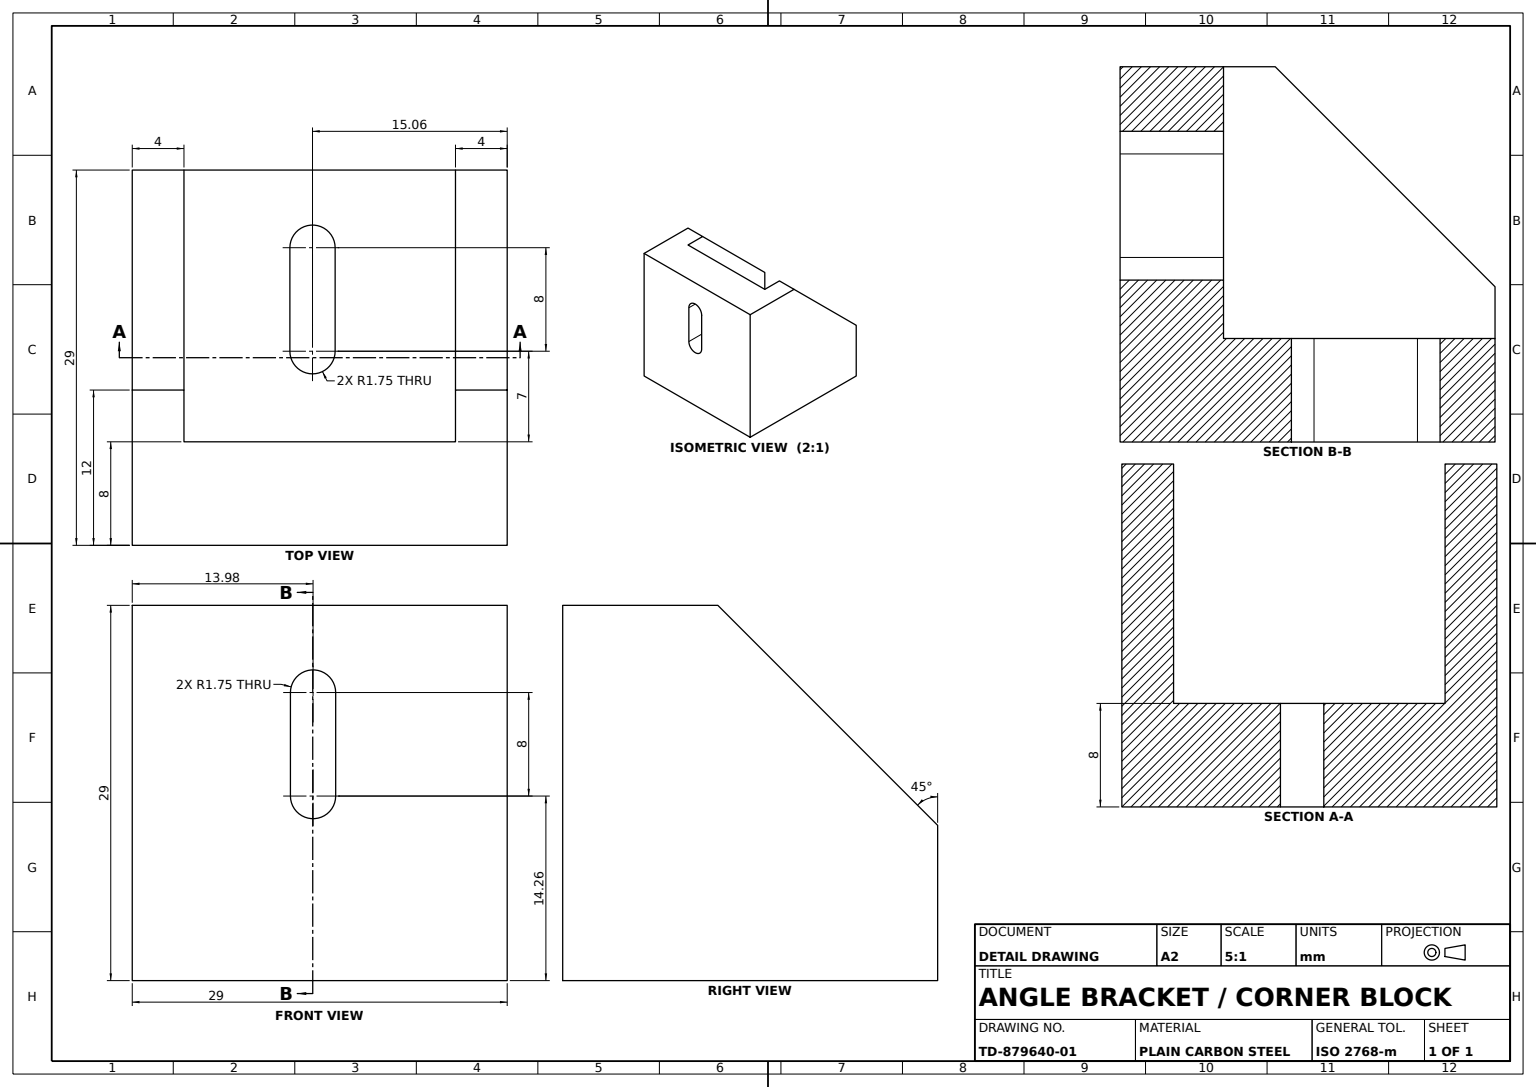
SolidWorks part; units mm, degrees
material "Plain Carbon Steel"
ref_plane "Front Plane" through (0, 0, 0) normal (0, 0, 1) x (1, 0, 0)
ref_plane "Top Plane" through (0, 0, 0) normal (0, 1, 0) x (1, 0, 0)
ref_plane "Right Plane" through (0, 0, 0) normal (1, 0, 0) x (0, 0, -1)
sketch "Base Plate Sketch" plane through (0, 0, 0) normal (0, 0, 1) x (1, 0, 0)
  line L0 (0, 0) -> (29, 0)
  line L1 (29, 0) -> (29, 29)
  line L2 (29, 29) -> (0, 29)
  line L3 (0, 29) -> (0, 0)
  dimension "D1" = 29
extrude "Base Plate 8mm" add sketch "Base Plate Sketch" along normal blind 8
sketch "Base Slot Sketch" plane through (0, 0, 8) normal (0, 0, 1) x (1, 0, 0)
  line L0 (12.2341, 22.2627) -> (12.2341, 14.2627)
  line L2 (15.7341, 14.2627) -> (15.7341, 22.2627)
  line L4 (29, 29) -> (0, 29) construction
  line L5 (0, 29) -> (0, 0) construction
  line L6 (0, 0) -> (29, 0) construction
  arc A0 (15.7341, 22.2627) -> (12.2341, 22.2627) centre (13.9841, 22.2627) ccw
  arc A1 (12.2341, 14.2627) -> (15.7341, 14.2627) centre (13.9841, 14.2627) ccw
  point P8 (15.7341, 18.2627)
  dimension "D1" = 3.5
  dimension "D2" = 3.5
  dimension "D4" = 1.75
  dimension "D3" = 10.7373
  dimension "D5" = 13.9841
  dimension "D6" = 14.2627
extrude "Base Slot 3.5mm" cut sketch "Base Slot Sketch" against normal blind 8
sketch "Upright Wall Sketch" plane through (0, 0, 0) normal (0, -1, 0) x (1, 0, 0)
  line L0 (29, 0) -> (29, -21)
  line L1 (29, -21) -> (0, -21)
  line L2 (0, -21) -> (0, 0)
  line L3 (0, 0) -> (29, 0)
  line L4 (0, 8) -> (29, 8) construction
  dimension "D1" = 29
extrude "Upright Wall 8mm" add sketch "Upright Wall Sketch" against normal blind 8
sketch "Wall Slot Sketch" plane through (0, 8, 0) normal (0, 1, 0) x (1, 0, 0)
  line L0 (12.1922, 15) -> (12.1922, 7)
  line L2 (15.6922, 7) -> (15.6922, 15)
  line L4 (0, 21) -> (29, 21) construction
  line L5 (29, 21) -> (29, 0) construction
  line L6 (29, 0) -> (0, 0) construction
  arc A0 (15.6922, 15) -> (12.1922, 15) centre (13.9422, 15) ccw
  arc A1 (12.1922, 7) -> (15.6922, 7) centre (13.9422, 7) ccw
  point P5 (15.6922, 11)
  dimension "D1" = 3.5
  dimension "D2" = 3.5
  dimension "D4" = 1.75
  dimension "D3" = 10
  dimension "D5" = 15.0578
  dimension "D6" = 7
extrude "Wall Slot 3.5mm" cut sketch "Wall Slot Sketch" against normal blind 8
sketch "Side Boss A Sketch" plane through (29, 0, 0) normal (1, 0, 0) x (0, 0, -1)
  line L0 (0, 29) -> (4, 29)
  line L1 (21, 8) -> (21, 12)
  line L2 (4, 29) -> (21, 12)
  line L3 (0, 29) -> (0, 8)
  line L4 (0, 8) -> (21, 8)
  dimension "D1" = 12
extrude "Side Boss A 4mm" add sketch "Side Boss A Sketch" against normal blind 4
sketch "Side Boss B Sketch" plane through (0, 0, 0) normal (-1, 0, 0) x (0, 0, 1)
  line L0 (0, 29) -> (-4, 29)
  line L1 (-21, 8) -> (-21, 12)
  line L2 (-21, 12) -> (-4, 29)
  line L9 (0, 29) -> (0, 8)
  line L10 (0, 8) -> (-21, 8)
  line L11 (-21, 8) -> (-21, 0)
  line L12 (-21, 0) -> (8, 0)
  line L13 (8, 0) -> (8, 29)
  line L14 (8, 29) -> (0, 29)
  line L15 (0, 29) -> (0, 8)
  line L16 (0, 8) -> (-21, 8)
  dimension "D1" = 0
  dimension "D2" = 4
extrude "Side Boss B 4mm" add sketch "Side Boss B Sketch" against normal blind 4
